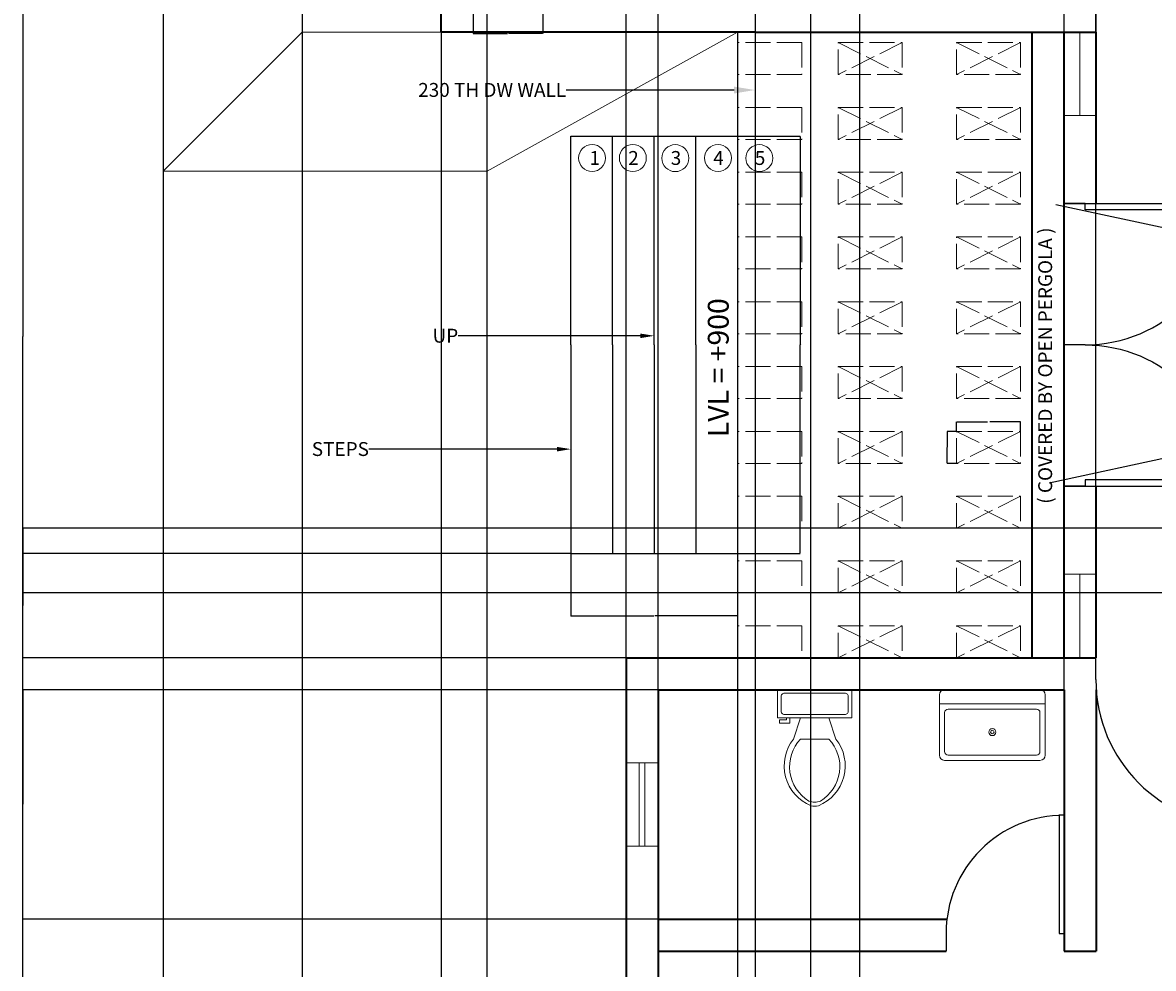
# Model space of a CAD drawing. Units: millimetres. Extents: x -8052 to 19968, y -37825 to -17505.
# Tile 2 of 10: x -8052 to 84, y -32209 to -25407. Entities that reach past the tile are written whole.
import ezdxf
from ezdxf import colors
from ezdxf.entities.mleader import LeaderData, LeaderLine
from ezdxf.math import Vec2, Vec3

# ---------------------------------------------------------------- set-up
doc = ezdxf.new("R2010")
doc.units = ezdxf.units.MM
doc.header["$MEASUREMENT"] = 0
doc.linetypes.add('ACAD_ISO02W100', pattern=[15, 12, -3])
for name, color, linetype, lineweight in [('A-ANNO-DIMS', 2, 'Continuous', 18), ('A-ANNO-SYMB', 7, 'Continuous', 18), ('A-ANNO-TEXT', 7, 'Continuous', 18), ('A-DOOR', 3, 'Continuous', 25), ('A-FLOR', 8, 'Continuous', 18), ('A-FLOR-FIXT', 9, 'Continuous', 18), ('A-FLOR-STRS', 7, 'Continuous', 25), ('A-GLAZ', 4, 'Continuous', 18), ('A-ROOF-OVHD', 8, 'ACAD_ISO02W100', 18), ('A-WALL', 7, 'Continuous', 35)]:
    doc.layers.add(name, color=color, linetype=linetype, lineweight=lineweight)
doc.styles.get("Standard").update_dxf_attribs({"font": 'arial.ttf'})
doc.dimstyles.get("Standard").update_dxf_attribs({"dimtxt": 1.054, "dimasz": 1.055, "dimexe": 0.18, "dimexo": 0.0625, "dimgap": 0.09, "dimtad": 0, "dimtih": 1, "dimtoh": 1, "dimdec": 4, "dimzin": 0, "dimdsep": 46, "dimtxsty": 'Standard', "dimcen": 0.09, "dimadec": 0, "dimazin": 0, "dimtfac": 1, "dimtdec": 4, "dimtofl": 0, "dimtmove": 0, "dimatfit": 3, "dimfxl": 1, "dimtolj": 1, "dimtzin": 0, "dimarcsym": 0})

# ---------------------------------------------------------------- blocks, each defined once
blk = doc.blocks.new('*U10')
for p, q in [((0, 0), (0, -6)), ((40, 0), (40, -6))]:
    blk.add_line(p, q)
blk.add_lwpolyline([(0, 0), (0, 40), (1.75, 40), (1.75, 0)], close=True)
blk.add_arc((0, 0), 40, 0, 90)
blk = doc.blocks.new('*U17')
for p, q in [((0, 0), (0, 6)), ((40, 0), (40, 6))]:
    blk.add_line(p, q)
blk.add_lwpolyline([(0, 0), (0, -40), (1.75, -40), (1.75, 0)], close=True)
blk.add_arc((0, 0), 40, 270, 0)
blk = doc.blocks.new('Sink-single - 30 in top')
blk.add_line((-15, -3.999996), (15, -3.999996))
for points in [[(-13.5, 0), (13.5, 0)], [(-15, -18.499996), (-15, -1.5)], [(15, -1.5), (15, -18.499996)], [(-12.5, -5.499996), (12.5, -5.499996)], [(-13.5, -17.499996), (-13.5, -6.499996)], [(13.5, -6.499996), (13.5, -17.499996)], [(12.5, -18.499996), (-12.5, -18.499996)], [(13.5, -19.999996), (-13.5, -19.999996)]]:
    blk.add_lwpolyline(points)
for radius in [1, 0.5]:
    blk.add_circle((0, -11.999996), radius)
for centre, radius, start, end in [((-13.5, -1.5), 1.5, 90, 180), ((13.5, -1.5), 1.5, 0, 90), ((-12.5, -6.499996), 1, 90, 180), ((12.5, -6.499996), 1, 0, 90), ((-13.5, -18.499996), 1.5, 180, 270), ((-12.5, -17.499996), 1, 180, 270), ((12.5, -17.499996), 1, 270, 0), ((13.5, -18.499996), 1.5, 270, 0)]:
    blk.add_arc(centre, radius, start, end)
blk = doc.blocks.new('Toilet - top')
for p, q in [((9.5, -6), (9.5, -2)), ((-10, -8.5), (-8, -8.5)), ((-10, -9.5), (-10, -8.5)), ((-7, -9.5), (-10, -9.5)), ((-8, -8.5), (-8, -8)), ((-7, -8), (-7, -9.5)), ((-4, -8), (-6, -14)), ((4, -8), (6, -14)), ((4, -14), (-4, -14))]:
    blk.add_line(p, q)
blk.add_lwpolyline([(10.5, -8), (10.5, 0), (-10.5, 0), (-10.5, -8)], close=True)
for points in [[(-9.5, -2), (-9.5, -6)], [(8.5, -1), (-8.5, -1)], [(-8.5, -7), (8.5, -7)]]:
    blk.add_lwpolyline(points)
for centre, radius, start, end in [((-8.62, -1.88), 0.884, 81.8699, 188.1301), ((8.62, -1.88), 0.884, 351.8699, 98.1301), ((-8.62, -6.12), 0.884, 171.8699, 278.1301), ((8.62, -6.12), 0.884, 261.8699, 8.1301), ((3.52, -21.58), 12.17, 141.4691, 247.9714), ((4.2, -21.82), 11.33, 136.3677, 238.9468), ((-3.52, -21.58), 12.17, 292.0284, 38.5307), ((-4.2, -21.82), 11.33, 301.053, 43.6321), ((0, -27.88), 4, 245.7318, 294.2682), ((0, -29), 4, 254.8605, 285.1395)]:
    blk.add_arc(centre, radius, start, end)
blk = doc.blocks.new('*U21')
for p, q in [((0, 0), (0, -6)), ((40, 0), (40, -6))]:
    blk.add_line(p, q)
blk.add_lwpolyline([(0, 0), (0, 40), (1.75, 40), (1.75, 0)], close=True)
blk.add_arc((0, 0), 40, 0, 90)
blk = doc.blocks.new('PERGOLA-CROSSED-MEMBER')
at = {"ltscale": 15}
for p, q in [((0, 230), (460, 0)), ((460, 230), (0, 0))]:
    blk.add_line(p, q, dxfattribs=at)
blk.add_lwpolyline([(0, 230), (460, 230), (460, 0), (0, 0)], close=True, dxfattribs=at)
blk = doc.blocks.new('PERGOLA-EDGE-MEMBER')
at = {"ltscale": 15}
for p, q in [((461.5, 230), (0, 230)), ((461.5, 230), (461.5, 0)), ((461.5, 0), (0, 0))]:
    blk.add_line(p, q, dxfattribs=at)
blk = doc.blocks.new('STAIR-SIDE-ENTRY-3000')
for p, q in [((0, 1500), (0, 3000)), ((0, 3000), (1200, 3000)), ((300, 1500), (300, 3000)), ((300, 1500), (300, 3000)), ((600, 1500), (600, 3000)), ((900, 1500), (900, 3000)), ((0, 1500), (0, 1500)), ((0, 1500), (0, 0)), ((300, 1500), (300, 0)), ((600, 1500), (600, 0)), ((900, 1500), (900, 0)), ((0, 0), (1200, 0))]:
    blk.add_line(p, q)
blk = doc.blocks.new('WIN-BATH-600')
for p, q in [((230, 600), (0, 600)), ((95, 600), (95, 0)), ((135, 600), (135, 0)), ((230, 0), (0, 0)), ((115, 0), (115, 0))]:
    blk.add_line(p, q)
blk = doc.blocks.new('WIN-SIDE-600')
for p, q in [((115, 0), (115, 600)), ((0, 0), (230, 0))]:
    blk.add_line(p, q)
blk = doc.blocks.new('*D60')
at = {"layer": 'A-ANNO-DIMS', "color": 0, "lineweight": -2, "transparency": 16777216}
for p, q in [((-2907.5, -26224.8), (-2457.3, -26224.8)), ((-2457.5, -26225.9), (-2457.5, -27724.2)), ((-2457.5, -29223.8), (-2457.5, -27725.5)), ((-2907.5, -29224.8), (-2457.3, -29224.8))]:
    blk.add_line(p, q, dxfattribs=at)
at = {"layer": 'A-ANNO-DIMS', "color": 0, "lineweight": 100, "transparency": 16777216}
for points in [[(-2457.7, -26225.9), (-2457.3, -26225.9), (-2457.5, -26224.8)], [(-2457.7, -29223.8), (-2457.3, -29223.8), (-2457.5, -29224.8)]]:
    blk.add_solid(points, dxfattribs=at)
at = {"layer": 'Defpoints', "color": 0, "lineweight": 100, "transparency": 16777216}
for p in [(-2907.5, -26224.8), (-2457.5, -26224.8), (-2907.5, -29224.8)]:
    blk.add_point(p, dxfattribs=at)
at = {"layer": 'A-ANNO-DIMS', "color": 0, "transparency": 16777216, "insert": (-2457.5, -27724.8), "char_height": 1.054, "attachment_point": 5}
blk.add_mtext('\\A1;ENTRY STEPS 3000 TYP.', dxfattribs=at)
blk = doc.blocks.new('*D61')
at = {"layer": 'A-ANNO-DIMS', "color": 0, "lineweight": -2, "transparency": 16777216}
for p, q in [((-4107.5, -29224.9), (-4107.5, -29675)), ((-2907.5, -29224.9), (-2907.5, -29675)), ((-4106.5, -29674.8), (-3510.9, -29674.8)), ((-2908.6, -29674.8), (-3504.1, -29674.8))]:
    blk.add_line(p, q, dxfattribs=at)
at = {"layer": 'A-ANNO-DIMS', "color": 0, "lineweight": 100, "transparency": 16777216}
for points in [[(-4106.5, -29674.7), (-4106.5, -29675), (-4107.5, -29674.8)], [(-2908.6, -29674.7), (-2908.6, -29675), (-2907.5, -29674.8)]]:
    blk.add_solid(points, dxfattribs=at)
at = {"layer": 'Defpoints', "color": 0, "lineweight": 100, "transparency": 16777216}
for p in [(-4107.5, -29224.8), (-2907.5, -29224.8), (-2907.5, -29674.8)]:
    blk.add_point(p, dxfattribs=at)
at = {"layer": 'A-ANNO-DIMS', "color": 0, "transparency": 16777216, "insert": (-3507.5, -29674.8), "char_height": 1.054, "attachment_point": 5}
blk.add_mtext('\\A1;1200 TYP.', dxfattribs=at)
blk = doc.blocks.new('*D69')
at = {"layer": 'A-ANNO-DIMS', "color": 0, "lineweight": -2, "transparency": 16777216}
for p, q in [((-4810, -25244.9), (-4810, -25485)), ((-4310, -25244.9), (-4310, -25485)), ((-4809, -25484.8), (-4563.1, -25484.8)), ((-4311.1, -25484.8), (-4557, -25484.8))]:
    blk.add_line(p, q, dxfattribs=at)
at = {"layer": 'A-ANNO-DIMS', "color": 0, "lineweight": 100, "transparency": 16777216}
for points in [[(-4809, -25484.7), (-4809, -25485), (-4810, -25484.8)], [(-4311.1, -25484.7), (-4311.1, -25485), (-4310, -25484.8)]]:
    blk.add_solid(points, dxfattribs=at)
at = {"layer": 'Defpoints', "color": 0, "lineweight": 100, "transparency": 16777216}
for p in [(-4810, -25244.8), (-4310, -25244.8), (-4310, -25484.8)]:
    blk.add_point(p, dxfattribs=at)
at = {"layer": 'A-ANNO-DIMS', "color": 0, "transparency": 16777216, "insert": (-4560, -25484.8), "char_height": 1.054, "attachment_point": 5}
blk.add_mtext('\\A1;500 TYP.', dxfattribs=at)
blk = doc.blocks.new('*D80')
at = {"layer": 'A-ANNO-DIMS', "color": 0, "lineweight": -2, "transparency": 16777216}
for p, q in [((-1331.3, -28346.8), (-1331.3, -28277.7)), ((-1330.3, -28277.9), (-1110.6, -28277.9)), ((-872.4, -28277.9), (-1092, -28277.9)), ((-871.3, -28346.8), (-871.3, -28277.7))]:
    blk.add_line(p, q, dxfattribs=at)
at = {"layer": 'A-ANNO-DIMS', "color": 0, "lineweight": 100, "transparency": 16777216}
for points in [[(-1330.3, -28277.7), (-1330.3, -28278.1), (-1331.3, -28277.9)], [(-872.4, -28277.7), (-872.4, -28278.1), (-871.3, -28277.9)]]:
    blk.add_solid(points, dxfattribs=at)
at = {"layer": 'Defpoints', "color": 0, "lineweight": 100, "transparency": 16777216}
for p in [(-871.3, -28277.9), (-1331.3, -28346.9), (-871.3, -28346.9)]:
    blk.add_point(p, dxfattribs=at)
at = {"layer": 'A-ANNO-DIMS', "color": 0, "transparency": 16777216, "insert": (-1101.3, -28277.9), "char_height": 1.054, "attachment_point": 5}
blk.add_mtext('\\A1;CROSS MEMBER 460 TYP.', dxfattribs=at)
blk = doc.blocks.new('*D81')
at = {"layer": 'A-ANNO-DIMS', "color": 0, "lineweight": -2, "transparency": 16777216}
for p, q in [((-1331.4, -28346.9), (-1400.5, -28346.9)), ((-1400.3, -28348), (-1400.3, -28461.3)), ((-1400.3, -28575.9), (-1400.3, -28462.5)), ((-1331.4, -28576.9), (-1400.5, -28576.9))]:
    blk.add_line(p, q, dxfattribs=at)
at = {"layer": 'A-ANNO-DIMS', "color": 0, "lineweight": 100, "transparency": 16777216}
for points in [[(-1400.5, -28348), (-1400.1, -28348), (-1400.3, -28346.9)], [(-1400.5, -28575.9), (-1400.1, -28575.9), (-1400.3, -28576.9)]]:
    blk.add_solid(points, dxfattribs=at)
at = {"layer": 'Defpoints', "color": 0, "lineweight": 100, "transparency": 16777216}
for p in [(-1400.3, -28346.9), (-1331.3, -28346.9), (-1331.3, -28576.9)]:
    blk.add_point(p, dxfattribs=at)
at = {"layer": 'A-ANNO-DIMS', "color": 0, "transparency": 16777216, "insert": (-1400.3, -28461.9), "char_height": 1.054, "attachment_point": 5}
blk.add_mtext('\\A1;230 TYP.', dxfattribs=at)
blk = doc.blocks.new('*D85')
at = {"layer": 'A-ANNO-DIMS', "color": 0, "lineweight": -2, "transparency": 16777216}
for p, q in [((-7040.1, -18514.8), (-8049.7, -18514.8)), ((-8049.5, -18515.9), (-8049.5, -27664.2)), ((-8049.5, -36813.8), (-8049.5, -27665.5)), ((-4710.1, -36814.8), (-8049.7, -36814.8))]:
    blk.add_line(p, q, dxfattribs=at)
at = {"layer": 'A-ANNO-DIMS', "color": 0, "lineweight": 100, "transparency": 16777216}
for points in [[(-8049.7, -18515.9), (-8049.3, -18515.9), (-8049.5, -18514.8)], [(-8049.7, -36813.8), (-8049.3, -36813.8), (-8049.5, -36814.8)]]:
    blk.add_solid(points, dxfattribs=at)
at = {"layer": 'Defpoints', "color": 0, "lineweight": 100, "transparency": 16777216}
for p in [(-7040, -18514.8), (-8049.5, -36814.8), (-4710, -36814.8)]:
    blk.add_point(p, dxfattribs=at)
at = {"layer": 'A-ANNO-DIMS', "color": 0, "transparency": 16777216, "insert": (-8049.5, -27664.8), "char_height": 1.05, "attachment_point": 5}
blk.add_mtext('\\A1;18300', dxfattribs=at)
blk = doc.blocks.new('*D86')
at = {"layer": 'A-ANNO-DIMS', "color": 0, "lineweight": -2, "transparency": 16777216}
for p, q in [((-7040, -18514.9), (-7040, -37824.5)), ((-6040, -19514.9), (-6040, -37824.5)), ((-7039, -37824.3), (-6541.6, -37824.3)), ((-6041.1, -37824.3), (-6538.4, -37824.3))]:
    blk.add_line(p, q, dxfattribs=at)
at = {"layer": 'A-ANNO-DIMS', "color": 0, "lineweight": 100, "transparency": 16777216}
for points in [[(-7039, -37824.2), (-7039, -37824.5), (-7040, -37824.3)], [(-6041.1, -37824.2), (-6041.1, -37824.5), (-6040, -37824.3)]]:
    blk.add_solid(points, dxfattribs=at)
at = {"layer": 'Defpoints', "color": 0, "lineweight": 100, "transparency": 16777216}
for p in [(-7040, -18514.8), (-6040, -19514.8), (-6040, -37824.3)]:
    blk.add_point(p, dxfattribs=at)
at = {"layer": 'A-ANNO-DIMS', "color": 0, "transparency": 16777216, "insert": (-6540, -37824.3), "char_height": 1.05, "attachment_point": 5}
blk.add_mtext('\\A1;1000', dxfattribs=at)
blk = doc.blocks.new('*D94')
at = {"layer": 'A-ANNO-DIMS', "color": 0, "lineweight": -2, "transparency": 16777216}
for p, q in [((-2780, -20744.9), (-2780, -37824.5)), ((-2030, -20744.9), (-2030, -37824.5)), ((-2779, -37824.3), (-2406.3, -37824.3)), ((-2031.1, -37824.3), (-2403.8, -37824.3))]:
    blk.add_line(p, q, dxfattribs=at)
at = {"layer": 'A-ANNO-DIMS', "color": 0, "lineweight": 100, "transparency": 16777216}
for points in [[(-2779, -37824.2), (-2779, -37824.5), (-2780, -37824.3)], [(-2031.1, -37824.2), (-2031.1, -37824.5), (-2030, -37824.3)]]:
    blk.add_solid(points, dxfattribs=at)
at = {"layer": 'Defpoints', "color": 0, "lineweight": 100, "transparency": 16777216}
for p in [(-2780, -20744.8), (-2030, -20744.8), (-2030, -37824.3)]:
    blk.add_point(p, dxfattribs=at)
at = {"layer": 'A-ANNO-DIMS', "color": 0, "transparency": 16777216, "insert": (-2405, -37824.3), "char_height": 1.05, "attachment_point": 5}
blk.add_mtext('\\A1;750', dxfattribs=at)
blk = doc.blocks.new('*D99')
at = {"layer": 'A-ANNO-DIMS', "color": 0, "lineweight": -2, "transparency": 16777216}
for p, q in [((-4710, -36814.8), (-4710, -17505.2)), ((-4709, -17505.3), (-4211.6, -17505.3)), ((-3711.1, -17505.3), (-4208.4, -17505.3)), ((-3710, -35814.8), (-3710, -17505.2))]:
    blk.add_line(p, q, dxfattribs=at)
at = {"layer": 'A-ANNO-DIMS', "color": 0, "lineweight": 100, "transparency": 16777216}
for points in [[(-4709, -17505.2), (-4709, -17505.5), (-4710, -17505.3)], [(-3711.1, -17505.2), (-3711.1, -17505.5), (-3710, -17505.3)]]:
    blk.add_solid(points, dxfattribs=at)
at = {"layer": 'Defpoints', "color": 0, "lineweight": 100, "transparency": 16777216}
for p in [(-3710, -17505.3), (-3710, -35814.8), (-4710, -36814.8)]:
    blk.add_point(p, dxfattribs=at)
at = {"layer": 'A-ANNO-DIMS', "color": 0, "transparency": 16777216, "insert": (-4210, -17505.3), "char_height": 1.05, "attachment_point": 5}
blk.add_mtext('\\A1;1000', dxfattribs=at)
blk = doc.blocks.new('*D103')
at = {"layer": 'A-ANNO-DIMS', "color": 0, "lineweight": -2, "transparency": 16777216}
for p, q in [((-3480, -35584.8), (-3480, -17505.2)), ((-3479, -17505.3), (-2931.6, -17505.3)), ((-2381.1, -17505.3), (-2928.4, -17505.3)), ((-2380, -35584.8), (-2380, -17505.2))]:
    blk.add_line(p, q, dxfattribs=at)
at = {"layer": 'A-ANNO-DIMS', "color": 0, "lineweight": 100, "transparency": 16777216}
for points in [[(-3479, -17505.2), (-3479, -17505.5), (-3480, -17505.3)], [(-2381.1, -17505.2), (-2381.1, -17505.5), (-2380, -17505.3)]]:
    blk.add_solid(points, dxfattribs=at)
at = {"layer": 'Defpoints', "color": 0, "lineweight": 100, "transparency": 16777216}
for p in [(-2380, -17505.3), (-3480, -35584.8), (-2380, -35584.8)]:
    blk.add_point(p, dxfattribs=at)
at = {"layer": 'A-ANNO-DIMS', "color": 0, "transparency": 16777216, "insert": (-2930, -17505.3), "char_height": 1.05, "attachment_point": 5}
blk.add_mtext('\\A1;1100', dxfattribs=at)
blk = doc.blocks.new('*D106')
at = {"layer": 'A-ANNO-DIMS', "color": 0, "lineweight": -2, "transparency": 16777216}
for p, q in [((-3480.1, -30204.8), (-8049.7, -30204.8)), ((-8049.5, -30205.9), (-8049.5, -31029.2)), ((-8049.5, -31853.8), (-8049.5, -31030.5)), ((-3480.1, -31854.8), (-8049.7, -31854.8))]:
    blk.add_line(p, q, dxfattribs=at)
at = {"layer": 'A-ANNO-DIMS', "color": 0, "lineweight": 100, "transparency": 16777216}
for points in [[(-8049.7, -30205.9), (-8049.3, -30205.9), (-8049.5, -30204.8)], [(-8049.7, -31853.8), (-8049.3, -31853.8), (-8049.5, -31854.8)]]:
    blk.add_solid(points, dxfattribs=at)
at = {"layer": 'Defpoints', "color": 0, "lineweight": 100, "transparency": 16777216}
for p in [(-3480, -30204.8), (-8049.5, -31854.8), (-3480, -31854.8)]:
    blk.add_point(p, dxfattribs=at)
at = {"layer": 'A-ANNO-DIMS', "color": 0, "transparency": 16777216, "insert": (-8049.5, -31029.8), "char_height": 1.05, "attachment_point": 5}
blk.add_mtext('\\A1;1650', dxfattribs=at)
blk = doc.blocks.new('*D107')
at = {"layer": 'A-ANNO-DIMS', "color": 0, "lineweight": -2, "transparency": 16777216}
for p, q in [((-3480, -30204.8), (-3480, -17505.2)), ((-3479, -17505.3), (-2021.1, -17505.3)), ((-558.6, -17505.3), (-2016.5, -17505.3)), ((-557.5, -30204.8), (-557.5, -17505.2))]:
    blk.add_line(p, q, dxfattribs=at)
at = {"layer": 'A-ANNO-DIMS', "color": 0, "lineweight": 100, "transparency": 16777216}
for points in [[(-3479, -17505.2), (-3479, -17505.5), (-3480, -17505.3)], [(-558.6, -17505.2), (-558.6, -17505.5), (-557.5, -17505.3)]]:
    blk.add_solid(points, dxfattribs=at)
at = {"layer": 'Defpoints', "color": 0, "lineweight": 100, "transparency": 16777216}
for p in [(-557.5, -17505.3), (-3480, -30204.8), (-557.5, -30204.8)]:
    blk.add_point(p, dxfattribs=at)
at = {"layer": 'A-ANNO-DIMS', "color": 0, "transparency": 16777216, "insert": (-2018.8, -17505.3), "char_height": 1.05, "attachment_point": 5}
blk.add_mtext('\\A1;2922.5', dxfattribs=at)
blk = doc.blocks.new('*D108')
at = {"layer": 'A-ANNO-DIMS', "color": 0, "lineweight": -2, "transparency": 16777216}
for p, q in [((-330, -29974.8), (-330, -17505.2)), ((-329, -17505.3), (3348.3, -17505.3)), ((7028.9, -17505.3), (3351.6, -17505.3)), ((7030, -29974.8), (7030, -17505.2))]:
    blk.add_line(p, q, dxfattribs=at)
at = {"layer": 'A-ANNO-DIMS', "color": 0, "lineweight": 100, "transparency": 16777216}
for points in [[(-329, -17505.2), (-329, -17505.5), (-330, -17505.3)], [(7028.9, -17505.2), (7028.9, -17505.5), (7030, -17505.3)]]:
    blk.add_solid(points, dxfattribs=at)
at = {"layer": 'Defpoints', "color": 0, "lineweight": 100, "transparency": 16777216}
for p in [(7030, -17505.3), (-330, -29974.8), (7030, -29974.8)]:
    blk.add_point(p, dxfattribs=at)
at = {"layer": 'A-ANNO-DIMS', "color": 0, "transparency": 16777216, "insert": (3350, -17505.3), "char_height": 1.05, "attachment_point": 5}
blk.add_mtext('\\A1;7360', dxfattribs=at)
blk = doc.blocks.new('*D110')
at = {"layer": 'A-ANNO-DIMS', "color": 0, "lineweight": -2, "transparency": 16777216}
for p, q in [((-4107.6, -29224.8), (-8049.7, -29224.8)), ((-8049.5, -29225.9), (-8049.5, -29599.2)), ((-8049.5, -29973.8), (-8049.5, -29600.5)), ((-2907.6, -29974.8), (-8049.7, -29974.8))]:
    blk.add_line(p, q, dxfattribs=at)
at = {"layer": 'A-ANNO-DIMS', "color": 0, "lineweight": 100, "transparency": 16777216}
for points in [[(-8049.7, -29225.9), (-8049.3, -29225.9), (-8049.5, -29224.8)], [(-8049.7, -29973.8), (-8049.3, -29973.8), (-8049.5, -29974.8)]]:
    blk.add_solid(points, dxfattribs=at)
at = {"layer": 'Defpoints', "color": 0, "lineweight": 100, "transparency": 16777216}
for p in [(-4107.5, -29224.8), (-8049.5, -29974.8), (-2907.5, -29974.8)]:
    blk.add_point(p, dxfattribs=at)
at = {"layer": 'A-ANNO-DIMS', "color": 0, "transparency": 16777216, "insert": (-8049.5, -29599.8), "char_height": 1.05, "attachment_point": 5}
blk.add_mtext('\\A1;750', dxfattribs=at)
blk = doc.blocks.new('*D111')
at = {"layer": 'A-ANNO-DIMS', "color": 0, "lineweight": -2, "transparency": 16777216}
for p, q in [((-560, -26708.8), (14099.7, -26708.8)), ((14099.5, -26709.9), (14099.5, -27724.2)), ((14099.5, -28739.8), (14099.5, -27725.5)), ((-560, -28740.8), (14099.7, -28740.8))]:
    blk.add_line(p, q, dxfattribs=at)
at = {"layer": 'A-ANNO-DIMS', "color": 0, "lineweight": 100, "transparency": 16777216}
for points in [[(14099.3, -26709.9), (14099.7, -26709.9), (14099.5, -26708.8)], [(14099.3, -28739.8), (14099.7, -28739.8), (14099.5, -28740.8)]]:
    blk.add_solid(points, dxfattribs=at)
at = {"layer": 'Defpoints', "color": 0, "lineweight": 100, "transparency": 16777216}
for p in [(-560, -26708.8), (-560, -28740.8), (14099.5, -28740.8)]:
    blk.add_point(p, dxfattribs=at)
at = {"layer": 'A-ANNO-DIMS', "color": 0, "transparency": 16777216, "insert": (14099.5, -27724.8), "char_height": 1.05, "attachment_point": 5}
blk.add_mtext('\\A1;2032', dxfattribs=at)
blk = doc.blocks.new('*D112')
at = {"layer": 'A-ANNO-DIMS', "color": 0, "lineweight": -2, "transparency": 16777216}
for p, q in [((8883.8, -29042.9), (-8049.7, -29042.9)), ((-8049.5, -29043.9), (-8049.5, -29275.2)), ((-8049.5, -29507.8), (-8049.5, -29276.5)), ((8883.8, -29508.9), (-8049.7, -29508.9))]:
    blk.add_line(p, q, dxfattribs=at)
at = {"layer": 'A-ANNO-DIMS', "color": 0, "lineweight": 100, "transparency": 16777216}
for points in [[(-8049.7, -29043.9), (-8049.3, -29043.9), (-8049.5, -29042.9)], [(-8049.7, -29507.8), (-8049.3, -29507.8), (-8049.5, -29508.9)]]:
    blk.add_solid(points, dxfattribs=at)
at = {"layer": 'Defpoints', "color": 0, "lineweight": 100, "transparency": 16777216}
for p in [(8883.8, -29042.9), (-8049.5, -29508.9), (8883.8, -29508.9)]:
    blk.add_point(p, dxfattribs=at)
at = {"layer": 'A-ANNO-DIMS', "color": 0, "transparency": 16777216, "insert": (-8049.5, -29275.9), "char_height": 1.05, "attachment_point": 5}
blk.add_mtext('\\A1;466', dxfattribs=at)
blk = doc.blocks.new('*D125')
at = {"layer": 'A-ANNO-DIMS', "color": 0, "lineweight": -2, "transparency": 16777216}
for p, q in [((-5040, -25474.9), (-5040, -37824.5)), ((-2907.5, -25474.9), (-2907.5, -37824.5)), ((-5039, -37824.3), (-3976.1, -37824.3)), ((-2908.6, -37824.3), (-3971.5, -37824.3))]:
    blk.add_line(p, q, dxfattribs=at)
at = {"layer": 'A-ANNO-DIMS', "color": 0, "lineweight": 100, "transparency": 16777216}
for points in [[(-5039, -37824.2), (-5039, -37824.5), (-5040, -37824.3)], [(-2908.6, -37824.2), (-2908.6, -37824.5), (-2907.5, -37824.3)]]:
    blk.add_solid(points, dxfattribs=at)
at = {"layer": 'Defpoints', "color": 0, "lineweight": 100, "transparency": 16777216}
for p in [(-5040, -25474.8), (-2907.5, -25474.8), (-2907.5, -37824.3)]:
    blk.add_point(p, dxfattribs=at)
at = {"layer": 'A-ANNO-DIMS', "color": 0, "transparency": 16777216, "insert": (-3973.8, -37824.3), "char_height": 1.05, "attachment_point": 5}
blk.add_mtext('\\A1;2132.5', dxfattribs=at)
blk = doc.blocks.new('*D133')
at = {"layer": 'A-ANNO-DIMS', "color": 0, "lineweight": -2, "transparency": 16777216}
for p, q in [((-617, -26716.3), (1188.8, -27099.5)), ((4201, -27738.9), (4201.2, -27738.9)), ((4201.1, -27739), (4201.1, -27738.8))]:
    blk.add_line(p, q, dxfattribs=at)
at = {"layer": 'A-ANNO-DIMS', "color": 0, "lineweight": 100, "transparency": 16777216}
blk.add_solid([(1188.8, -27099.4), (1188.7, -27099.7), (1189.8, -27099.7)], dxfattribs=at)
at = {"layer": 'Defpoints', "color": 0, "lineweight": 100, "transparency": 16777216}
for p in [(1189.8, -27099.7), (4201.1, -27738.9)]:
    blk.add_point(p, dxfattribs=at)
at = {"layer": 'A-ANNO-DIMS', "color": 0, "transparency": 16777216, "insert": (-619.8, -26716.3), "char_height": 1.054, "attachment_point": 5}
blk.add_mtext('\\A1;R3078.4', dxfattribs=at)
blk = doc.blocks.new('*D134')
at = {"layer": 'A-ANNO-DIMS', "color": 0, "lineweight": -2, "transparency": 16777216}
for p, q in [((3872.2, -27738.9), (3872.4, -27738.9)), ((3872.3, -27739), (3872.3, -27738.8)), ((-666.8, -28716.5), (1034.3, -28350.1))]:
    blk.add_line(p, q, dxfattribs=at)
at = {"layer": 'A-ANNO-DIMS', "color": 0, "lineweight": 100, "transparency": 16777216}
blk.add_solid([(1034.3, -28350), (1034.4, -28350.3), (1035.4, -28349.9)], dxfattribs=at)
at = {"layer": 'Defpoints', "color": 0, "lineweight": 100, "transparency": 16777216}
for p in [(3872.3, -27738.9), (1035.4, -28349.9)]:
    blk.add_point(p, dxfattribs=at)
at = {"layer": 'A-ANNO-DIMS', "color": 0, "transparency": 16777216, "insert": (-668.9, -28716.5), "char_height": 1.05, "attachment_point": 5}
blk.add_mtext('\\A1;R2902', dxfattribs=at)

msp = doc.modelspace()

# ---------------------------------------------------------------- linework, layer by layer
at = {"layer": 'A-ANNO-SYMB'}
for centre in [(-3954.392, -26381.051), (-3661.31, -26381.051), (-3355.961, -26381.938), (-3048.396, -26380.846), (-2750.485, -26381.699)]:
    msp.add_circle(centre, 97, dxfattribs=at)
at = {"layer": 'A-DOOR'}
msp.add_line((-330.021, -25317.343), (-330.021, -25474.843), dxfattribs=at)
at = {"layer": 'A-FLOR'}
for p, q in [((-7040.021, -26474.843), (-7040.021, -20744.843)), ((-6040.021, -25474.843), (-6040.021, -25244.843)), ((-6040.021, -25474.843), (-7040.021, -26474.843)), ((-6040.021, -25474.843), (-5040.021, -25474.843)), ((-4710.021, -26474.843), (-2907.521, -25474.843)), ((-2907.521, -25474.843), (-2907.521, -29974.843)), ((-4710.021, -26474.843), (-7040.021, -26474.843)), ((-4710.021, -26474.843), (-4710.021, -36814.843))]:
    msp.add_line(p, q, dxfattribs=at)
at = {"layer": 'A-WALL'}
for p, q in [((-5040.021, -25474.843), (-5040.021, -25244.843)), ((-4810.021, -25474.843), (-5040.021, -25474.843)), ((-3010.021, -25474.843), (-4810.021, -25474.843)), ((-2780.021, -25474.843), (-3010.021, -25474.843)), ((-2780.021, -25474.843), (-330.021, -25474.843)), ((-790.021, -25474.843), (-790.021, -29974.843)), ((-560.021, -25474.843), (-560.021, -29974.843)), ((-330.021, -25474.843), (-330.021, -26708.843)), ((-330.021, -28740.843), (-330.021, -29974.843)), ((-3710.021, -29974.843), (-330.021, -29974.843)), ((-3710.021, -29974.843), (-3710.021, -35814.843)), ((-3480.021, -30204.843), (-557.515, -30204.843)), ((-3480.021, -30204.843), (-3480.021, -35584.843)), ((-557.515, -30204.843), (-557.515, -32084.843)), ((-327.515, -30204.843), (-327.515, -32084.843)), ((-3480.021, -31854.843), (-1401.312, -31854.843)), ((-3480.021, -32084.843), (-1407.515, -32084.843)), ((-557.515, -32084.843), (-327.515, -32084.843))]:
    msp.add_line(p, q, dxfattribs=at)

# ---------------------------------------------------------------- block references
at = {"layer": 'A-DOOR'}
for name, p, xscale, yscale, zscale, rotation in [('*U21', (-407.621, -26708.843), 25.4, 25.4, 25.4, 270), ('*U21', (-407.621, -28740.843), -25.4, 25.4, 25.4, 270), ('*U10', (719.979, -30132.343), 26.25, 26.25, 26.25, 180), ('*U17', (-557.515, -31957.343), 21.25, 21.25, 21.25, 180)]:
    msp.add_blockref(name, p, dxfattribs=dict(at, xscale=xscale, yscale=yscale, zscale=zscale, rotation=rotation))
at = {"layer": 'A-FLOR-FIXT', "xscale": 25.4, "yscale": 25.4, "zscale": 25.4}
for name, p in [('Toilet - top', (-2352.721, -30204.843)), ('Sink-single - 30 in top', (-1074.859, -30204.843))]:
    msp.add_blockref(name, p, dxfattribs=at)
at = {"layer": 'A-FLOR-STRS'}
msp.add_blockref('STAIR-SIDE-ENTRY-3000', (-4107.521, -29224.843), dxfattribs=at)
at = {"layer": 'A-GLAZ'}
for name, p in [('WIN-SIDE-600', (-560.021, -26074.843)), ('WIN-BATH-600', (-3710.021, -31329.843))]:
    msp.add_blockref(name, p, dxfattribs=at)
at = {"layer": 'A-GLAZ', "rotation": 180}
msp.add_blockref('WIN-SIDE-600', (-330.02, -29374.843), dxfattribs=at)
at = {"layer": 'A-ROOF-OVHD'}
for name, p in [('PERGOLA-EDGE-MEMBER', (-2907.521, -25781.045)), ('PERGOLA-CROSSED-MEMBER', (-2183.879, -25781.045)), ('PERGOLA-CROSSED-MEMBER', (-1331.316, -25781.045)), ('PERGOLA-EDGE-MEMBER', (-2907.521, -26247.023)), ('PERGOLA-CROSSED-MEMBER', (-2183.879, -26247.023)), ('PERGOLA-CROSSED-MEMBER', (-1331.316, -26247.023)), ('PERGOLA-EDGE-MEMBER', (-2907.521, -26713)), ('PERGOLA-CROSSED-MEMBER', (-2183.879, -26713)), ('PERGOLA-CROSSED-MEMBER', (-1331.316, -26713)), ('PERGOLA-EDGE-MEMBER', (-2907.521, -27178.978)), ('PERGOLA-CROSSED-MEMBER', (-2183.879, -27178.978)), ('PERGOLA-CROSSED-MEMBER', (-1331.316, -27178.978)), ('PERGOLA-EDGE-MEMBER', (-2907.521, -27644.955)), ('PERGOLA-CROSSED-MEMBER', (-2183.879, -27644.955)), ('PERGOLA-CROSSED-MEMBER', (-1331.316, -27644.955)), ('PERGOLA-EDGE-MEMBER', (-2907.521, -28110.933)), ('PERGOLA-CROSSED-MEMBER', (-2183.879, -28110.933)), ('PERGOLA-CROSSED-MEMBER', (-1331.316, -28110.933)), ('PERGOLA-EDGE-MEMBER', (-2907.521, -28576.91)), ('PERGOLA-CROSSED-MEMBER', (-2183.879, -28576.91)), ('PERGOLA-CROSSED-MEMBER', (-1331.316, -28576.91)), ('PERGOLA-EDGE-MEMBER', (-2907.521, -29042.888)), ('PERGOLA-CROSSED-MEMBER', (-2183.879, -29042.888)), ('PERGOLA-CROSSED-MEMBER', (-1331.316, -29042.888)), ('PERGOLA-EDGE-MEMBER', (-2907.521, -29508.865)), ('PERGOLA-CROSSED-MEMBER', (-2183.879, -29508.865)), ('PERGOLA-CROSSED-MEMBER', (-1331.316, -29508.865)), ('PERGOLA-EDGE-MEMBER', (-2907.521, -29974.843)), ('PERGOLA-CROSSED-MEMBER', (-2183.879, -29974.843)), ('PERGOLA-CROSSED-MEMBER', (-1331.316, -29974.843))]:
    msp.add_blockref(name, p, dxfattribs=at)

# ---------------------------------------------------------------- texts
at = {"layer": 'A-ANNO-TEXT', "char_height": 100, "attachment_point": 1}
for s, insert in [('1', (-3972.809, -26330.846)), ('2', (-3694.427, -26330.846)), ('3', (-3388.704, -26330.846)), ('4', (-3082.98, -26330.846)), ('5', (-2783.636, -26330.846))]:
    msp.add_mtext_dynamic_manual_height_columns(s, width=159.07556, gutter_width=1, heights=[0], dxfattribs=dict(at, insert=insert))
at = {"layer": 'A-ANNO-TEXT', "attachment_point": 1, "rotation": 90}
for s, width, insert, char_height in [('( COVERED BY OPEN PERGOLA )', 2294.41831, (-744.242, -28867.616), 100), ('LVL = +900', 1598.33979, (-3121.578, -28388.9), 150)]:
    msp.add_mtext_dynamic_manual_height_columns(s, width=width, gutter_width=1, heights=[0], dxfattribs=dict(at, insert=insert, char_height=char_height))

# ---------------------------------------------------------------- dimensions: what is measured, and where the dimension line sits
at = {"layer": 'A-ANNO-DIMS'}
for base, p1, p2, override, picture, middle in [((-3710.021, -17505.343), (-4710.021, -36814.843), (-3710.021, -35814.843), {"dimdec": 0, "dimlfac": 1, "dimrnd": 0, "dimzin": 0, "dimdsep": 46, "dimlunit": 2}, '*D99', (-4210.021, -17505.343)), ((-2380.021, -17505.343), (-3480.021, -35584.843), (-2380.021, -35584.843), {"dimdec": 0, "dimlfac": 1, "dimrnd": 0, "dimzin": 0, "dimdsep": 46, "dimlunit": 2}, '*D103', (-2930.021, -17505.343)), ((-557.515, -17505.343), (-3480.021, -30204.843), (-557.515, -30204.843), {"dimdec": 1, "dimlfac": 1, "dimrnd": 0, "dimzin": 0, "dimdsep": 46, "dimlunit": 2}, '*D107', (-2018.768, -17505.343)), ((7029.979, -17505.343), (-330.021, -29974.843), (7029.979, -29974.843), {"dimdec": 0, "dimlfac": 1, "dimrnd": 0, "dimzin": 0, "dimdsep": 46, "dimlunit": 2}, '*D108', (3349.979, -17505.343)), ((-6040.021, -37824.343), (-7040.021, -18514.843), (-6040.021, -19514.843), {"dimdec": 0, "dimlfac": 1, "dimrnd": 0, "dimzin": 0, "dimdsep": 46, "dimlunit": 2}, '*D86', (-6540.021, -37824.343)), ((-2030.021, -37824.343), (-2780.021, -20744.843), (-2030.021, -20744.843), {"dimdec": 0, "dimlfac": 1, "dimrnd": 0, "dimzin": 0, "dimdsep": 46, "dimlunit": 2}, '*D94', (-2405.021, -37824.343)), ((-2907.521, -37824.343), (-5040.021, -25474.843), (-2907.521, -25474.843), {"dimdec": 1, "dimlfac": 1, "dimrnd": 0, "dimzin": 0, "dimdsep": 46, "dimlunit": 2}, '*D125', (-3973.771, -37824.343))]:
    dim = msp.add_linear_dim(base=base, p1=p1, p2=p2, dimstyle='Standard', override=override, dxfattribs=at)
    dim.commit()
    dim.dimension.update_dxf_attribs({"geometry": picture, "text_midpoint": middle})
for base, p1, p2, picture, middle in [((-8049.521, -36814.843), (-7040.021, -18514.843), (-4710.021, -36814.843), '*D85', (-8049.521, -27664.843)), ((14099.479, -28740.843), (-560.021, -26708.843), (-560.021, -28740.843), '*D111', (14099.479, -27724.843)), ((-8049.521, -29508.866), (8883.837, -29042.888), (8883.837, -29508.866), '*D112', (-8049.521, -29275.877)), ((-8049.521, -29974.843), (-4107.521, -29224.843), (-2907.521, -29974.843), '*D110', (-8049.521, -29599.843)), ((-8049.521, -31854.843), (-3480.021, -30204.843), (-3480.021, -31854.843), '*D106', (-8049.521, -31029.843))]:
    dim = msp.add_linear_dim(base=base, p1=p1, p2=p2, angle=90, dimstyle='Standard', override={"dimdec": 0, "dimlfac": 1, "dimrnd": 0, "dimzin": 0, "dimdsep": 46, "dimlunit": 2}, dxfattribs=at)
    dim.commit()
    dim.dimension.update_dxf_attribs({"geometry": picture, "text_midpoint": middle})
for base, p1, p2, text, picture, middle in [((-4310.021, -25484.843), (-4810.021, -25244.843), (-4310.021, -25244.843), '<> TYP.', '*D69', (-4560.021, -25484.843)), ((-871.316, -28277.91), (-1331.316, -28346.91), (-871.316, -28346.91), 'CROSS MEMBER <> TYP.', '*D80', (-1101.316, -28277.91)), ((-2907.521, -29674.843), (-4107.521, -29224.843), (-2907.521, -29224.843), '<> TYP.', '*D61', (-3507.521, -29674.843))]:
    dim = msp.add_linear_dim(base=base, p1=p1, p2=p2, text=text, dimstyle='Standard', override={"dimdec": 0, "dimlfac": 1, "dimrnd": 0, "dimzin": 0, "dimdsep": 46, "dimlunit": 2}, dxfattribs=at)
    dim.commit()
    dim.dimension.update_dxf_attribs({"geometry": picture, "text_midpoint": middle})
for base, p1, p2, text, picture, middle in [((-2457.521, -26224.843), (-2907.521, -29224.843), (-2907.521, -26224.843), 'ENTRY STEPS <> TYP.', '*D60', (-2457.521, -27724.843)), ((-1400.316, -28346.91), (-1331.316, -28576.91), (-1331.316, -28346.91), '<> TYP.', '*D81', (-1400.316, -28461.91))]:
    dim = msp.add_linear_dim(base=base, p1=p1, p2=p2, angle=90, text=text, dimstyle='Standard', override={"dimdec": 0, "dimlfac": 1, "dimrnd": 0, "dimzin": 0, "dimdsep": 46, "dimlunit": 2}, dxfattribs=at)
    dim.commit()
    dim.dimension.update_dxf_attribs({"geometry": picture, "text_midpoint": middle})
for center, mpoint, override, picture, middle in [((4201.122, -27738.889), (1189.804, -27099.746), {"dimdec": 1, "dimlfac": 1, "dimrnd": 0, "dimzin": 0, "dimdsep": 46, "dimlunit": 2}, '*D133', (-616.987, -26716.26)), ((3872.273, -27738.889), (1035.381, -28349.918), {"dimdec": 0, "dimlfac": 1, "dimrnd": 0, "dimzin": 0, "dimdsep": 46, "dimlunit": 2}, '*D134', (-666.755, -28716.535))]:
    dim = msp.add_radius_dim(center=center, mpoint=mpoint, dimstyle='Standard', override=override, dxfattribs=at)
    dim.commit()
    dim.dimension.update_dxf_attribs({"geometry": picture, "text_midpoint": middle, "dimtype": 164})

# ---------------------------------------------------------------- leaders
at = {"layer": 'A-ANNO-TEXT'}
ml = msp.add_multileader_mtext('Standard', dxfattribs=at)
ml.set_content('230 TH DW WALL', color=256)
ml.set_leader_properties()
ml.build(insert=Vec2(0, 0))
ml.multileader.update_dxf_attribs({"dogleg_length": 0.36, "arrow_head_size": 150})
ctx = ml.context
ctx.base_point, ctx.char_height, ctx.arrow_head_size, ctx.landing_gap_size, ctx.plane_origin = Vec3(-5281.153, -25892.244), 100, 150, 0.09, Vec3(-2782.742, -25892.244)
ctx.text_align_type = 2
notes = []
notes.append((ctx, [(0, (1, 1, 0), (-4140.777, -25892.244), (-1, 0), 0.36, [(0, [(-2782.742, -25892.244)], 0, [])])]))
ctx.mtext.insert, ctx.mtext.alignment, ctx.mtext.flow_direction = Vec3(-4141.227, -25841.357), 3, 5
ml = msp.add_multileader_mtext('Standard', dxfattribs=at)
ml.set_content('\\pxt1;UP', color=256)
ml.set_leader_properties()
ml.build(insert=Vec2(0, 0))
ml.multileader.update_dxf_attribs({"dogleg_length": 0.36, "arrow_head_size": 100})
ctx = ml.context
ctx.base_point, ctx.char_height, ctx.arrow_head_size, ctx.landing_gap_size, ctx.plane_origin = Vec3(-5094.766, -27659.789), 100, 100, 0.09, Vec3(-3507.521, -27659.789)
ctx.text_align_type = 2
notes.append((ctx, [(0, (1, 1, 0), (-4917.214, -27659.789), (-1, 0), 0.36, [(0, [(-3507.521, -27659.789)], 0, [])])]))
ctx.mtext.insert, ctx.mtext.width, ctx.mtext.alignment, ctx.mtext.flow_direction = Vec3(-4917.664, -27608.937), 0.34019, 3, 5
ml = msp.add_multileader_mtext('Standard', dxfattribs=at)
ml.set_content('STEPS', color=256)
ml.set_leader_properties()
ml.build(insert=Vec2(0, 0))
ml.multileader.update_dxf_attribs({"dogleg_length": 0.36, "arrow_head_size": 100})
ctx = ml.context
ctx.base_point, ctx.char_height, ctx.arrow_head_size, ctx.landing_gap_size, ctx.plane_origin = Vec3(-6004.696, -28474.843), 100, 100, 0.09, Vec3(-4107.521, -28474.843)
ctx.text_align_type = 2
notes.append((ctx, [(0, (1, 1, 0), (-5559.681, -28474.843), (-1, 0), 0.36, [(0, [(-4107.521, -28474.843)], 0, [])])]))
ctx.mtext.insert, ctx.mtext.alignment, ctx.mtext.flow_direction = Vec3(-5560.131, -28423.99), 3, 5
for ctx, leaders in notes:
    for number, flags, end, landing, length, lines in leaders:
        leader = LeaderData()
        leader.index, (leader.has_last_leader_line, leader.has_dogleg_vector, leader.attachment_direction) = number, flags
        leader.last_leader_point, leader.dogleg_vector, leader.dogleg_length = Vec3(end), Vec3(landing), length
        for number, points, colour, breaks in lines:
            line = LeaderLine()
            line.index, line.vertices, line.color, line.breaks = number, Vec3.list(points), colors.encode_raw_color(colour), breaks
            leader.lines.append(line)
        ctx.leaders.append(leader)

doc.saveas('drawing.dxf')
